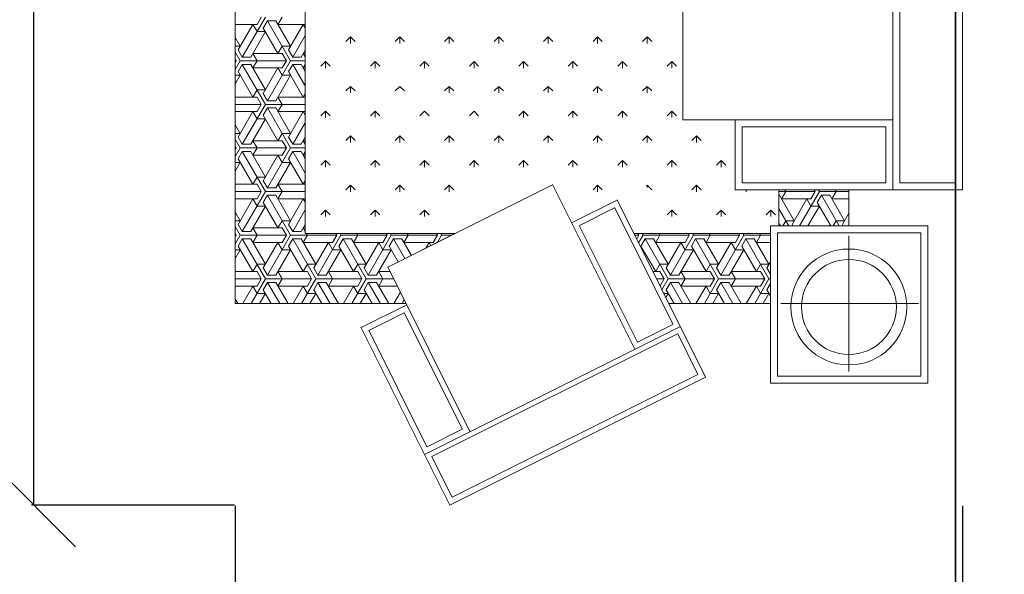
# Model space of a CAD drawing. Units: inches. Extents: x -1198 to -69, y -512 to 437.
# Tile 44 of 50: x -444 to -373, y 5 to 45. Entities that reach past the tile are written whole.
import ezdxf

# ---------------------------------------------------------------- set-up
doc = ezdxf.new("R2010")
doc.units = ezdxf.units.IN
doc.header["$MEASUREMENT"] = 0
for name, color, linetype, lineweight in [('A-ANNO-DIMS', 2, 'Continuous', 18), ('A-FURN', 60, 'Continuous', 18), ('A-WALL', 7, 'Continuous', 35)]:
    doc.layers.add(name, color=color, linetype=linetype, lineweight=lineweight)
doc.styles.get("Standard").update_dxf_attribs({"font": 'arial.ttf'})
doc.dimstyles.get("Standard").update_dxf_attribs({"dimtxt": 6, "dimasz": 6, "dimexe": 0.18, "dimexo": 0.0625, "dimgap": 0.09, "dimtad": 0, "dimtih": 1, "dimtoh": 1, "dimdec": 0, "dimzin": 0, "dimdsep": 46, "dimlunit": 4, "dimtxsty": 'Standard', "dimblk": 'OBLIQUE', "dimcen": 0.09, "dimadec": 0, "dimazin": 0, "dimtfac": 1, "dimtdec": 0, "dimtofl": 0, "dimtmove": 0, "dimatfit": 3, "dimfxl": 1, "dimtolj": 1, "dimtzin": 0, "dimarcsym": 0})

# ---------------------------------------------------------------- blocks, each defined once
blk = doc.blocks.new('A$C3B9F700E')
for p, q in [((736.9, 2080, -685.7), (2936.9, 2080, -685.7)), ((756.9, 2060, -685.7), (2916.9, 2060, -685.7)), ((2916.9, 2060, -685.7), (2916.9, 1900, -685.7)), ((2936.9, 2080, -685.7), (2936.9, 1430, -685.7)), ((2936.9, 2080, -685.7), (2936.9, 1880, -685.7)), ((3489.8, 1980.6, -685.7), (3039.8, 1980.6, -685.7)), ((3039.8, 1980.6, -685.7), (3039.8, 1530.6, -685.7)), ((3489.8, 1530.6, -685.7), (3489.8, 1980.6, -685.7)), ((3469.8, 1960.6, -685.7), (3059.8, 1960.6, -685.7)), ((3059.8, 1960.6, -685.7), (3059.8, 1550.6, -685.7)), ((3262.1, 1953.9, -685.7), (3262.1, 1560.5, -685.7)), ((3469.8, 1550.6, -685.7), (3469.8, 1960.6, -685.7)), ((2916.9, 1900, -685.7), (756.9, 1900, -685.7)), ((2936.9, 1880, -685.7), (736.9, 1880, -685.7)), ((2936.9, 1880, -685.7), (736.9, 1880, -685.7)), ((2736.9, 1880, -685.7), (2736.9, 1280, -685.7)), ((2736.9, 1430, -685.7), (2736.9, 1880, -685.7)), ((2736.9, 1880, -685.7), (2936.9, 1880, -685.7)), ((2756.9, 1450, -685.7), (2756.9, 1860, -685.7)), ((2756.9, 1860, -685.7), (2916.9, 1860, -685.7)), ((2916.9, 1860, -685.7), (2916.9, 1450, -685.7)), ((2936.9, 1880, -685.7), (2936.9, 1430, -685.7)), ((2936.9, 1754.8, -685.7), (3039.8, 1754.8, -685.7)), ((2936.9, 1554.8, -685.7), (2936.9, 1754.8, -685.7)), ((2936.9, 1754.8, -685.7), (3039.8, 1754.8, -685.7)), ((2941.9, 1670.3, -685.7), (2941.9, 1754.8, -685.7)), ((2962.7, 1754.8, -685.7), (2962.7, 1706.3, -685.7)), ((3035.5, 1736.3, -685.7), (3003.4, 1754.8, -685.7)), ((3039.8, 1754.8, -685.7), (3039.8, 1554.8, -685.7)), ((3456.2, 1754.8, -685.7), (3068, 1754.8, -685.7)), ((2941.9, 1718.3, -685.7), (2936.9, 1715.4, -685.7)), ((2941.9, 1718.3, -685.7), (2962.7, 1706.3, -685.7)), ((2952.3, 1700.3, -685.7), (3025.1, 1742.3, -685.7)), ((3039.8, 1726.8, -685.7), (2952.3, 1676.3, -685.7)), ((3025.1, 1718.3, -685.7), (3025.1, 1742.3, -685.7)), ((3025.1, 1718.3, -685.7), (3039.8, 1709.8, -685.7)), ((3039.8, 1738.8, -685.7), (3035.5, 1736.3, -685.7)), ((2952.3, 1676.3, -685.7), (2952.3, 1700.3, -685.7)), ((2973.1, 1664.3, -685.7), (3039.8, 1702.8, -685.7)), ((2941.9, 1670.3, -685.7), (2936.9, 1667.4, -685.7)), ((2941.9, 1670.3, -685.7), (3039.8, 1613.8, -685.7)), ((2952.3, 1676.3, -685.7), (2973.1, 1664.3, -685.7)), ((3039.8, 1637.8, -685.7), (2983.5, 1670.3, -685.7)), ((2983.5, 1646.3, -685.7), (2983.5, 1670.3, -685.7)), ((2941.9, 1658.3, -685.7), (2936.9, 1655.4, -685.7)), ((2941.9, 1658.3, -685.7), (2962.7, 1646.3, -685.7)), ((2941.9, 1554.8, -685.7), (2941.9, 1658.3, -685.7)), ((2962.7, 1646.3, -685.7), (2962.7, 1562.3, -685.7)), ((2983.5, 1646.3, -685.7), (2962.7, 1634.3, -685.7)), ((3035.5, 1592.3, -685.7), (2962.7, 1634.3, -685.7)), ((2952.3, 1556.3, -685.7), (3025.1, 1598.3, -685.7)), ((3039.8, 1582.8, -685.7), (2991.3, 1554.8, -685.7)), ((3025.1, 1574.3, -685.7), (3025.1, 1598.3, -685.7)), ((3039.8, 1594.8, -685.7), (3035.5, 1592.3, -685.7)), ((2941.9, 1574.3, -685.7), (2936.9, 1571.4, -685.7)), ((3039.8, 1554.8, -685.7), (2936.9, 1554.8, -685.7)), ((2936.9, 1554.8, -685.7), (3039.8, 1554.8, -685.7)), ((2941.9, 1574.3, -685.7), (2962.7, 1562.3, -685.7)), ((2952.3, 1554.8, -685.7), (2952.3, 1556.3, -685.7)), ((3025.1, 1574.3, -685.7), (3039.8, 1565.8, -685.7)), ((3032.8, 1554.8, -685.7), (3039.8, 1558.8, -685.7)), ((3059.8, 1550.6, -685.7), (3469.8, 1550.6, -685.7)), ((2994.6, 1531.3, -685.7), (3007.9, 1544.5, -685.7)), ((2994.6, 1531.3, -685.7), (3013.4, 1531.3, -685.7)), ((2994.6, 1531.3, -685.7), (3007.9, 1518, -685.7)), ((3039.8, 1530.6, -685.7), (3489.8, 1530.6, -685.7)), ((3062.1, 1140.2, -685.7), (3062.1, 1530.6, -685.7)), ((3062.1, 1530.6, -685.7), (3062.1, 1140.2, -685.7)), ((3062.1, 1530.6, -685.7), (3262.1, 1530.6, -685.7)), ((3066.6, 1454.3, -685.7), (3066.6, 1530.6, -685.7)), ((3077, 1484.3, -685.7), (3149.8, 1526.3, -685.7)), ((3191.3, 1526.3, -685.7), (3077, 1460.3, -685.7)), ((3087.4, 1530.6, -685.7), (3087.4, 1490.3, -685.7)), ((3160.2, 1520.3, -685.7), (3142.3, 1530.6, -685.7)), ((3149.8, 1502.3, -685.7), (3149.8, 1526.3, -685.7)), ((3178, 1530.6, -685.7), (3160.2, 1520.3, -685.7)), ((3191.3, 1526.3, -685.7), (3191.3, 1530.6, -685.7)), ((3191.3, 1526.3, -685.7), (3262.1, 1485.5, -685.7)), ((3204.7, 1530.6, -685.7), (3222.5, 1520.3, -685.7)), ((3222.5, 1520.3, -685.7), (3240.3, 1530.6, -685.7)), ((3262.1, 1509.5, -685.7), (3232.9, 1526.3, -685.7)), ((3232.9, 1502.3, -685.7), (3232.9, 1526.3, -685.7)), ((3262.1, 1530.6, -685.7), (3262.1, 1240.1, -685.7)), ((3262.1, 1530.6, -685.7), (3262.1, 1240.1, -685.7)), ((3066.6, 1502.3, -685.7), (3062.1, 1499.7, -685.7)), ((3066.6, 1502.3, -685.7), (3087.4, 1490.3, -685.7)), ((3149.8, 1502.3, -685.7), (3170.6, 1490.3, -685.7)), ((3191.3, 1514.3, -685.7), (3170.6, 1502.3, -685.7)), ((3170.6, 1502.3, -685.7), (3170.6, 1418.3, -685.7)), ((3191.3, 1382.3, -685.7), (3191.3, 1514.3, -685.7)), ((3191.3, 1514.3, -685.7), (3212.1, 1502.3, -685.7)), ((3212.1, 1502.3, -685.7), (3212.1, 1418.3, -685.7)), ((3232.9, 1502.3, -685.7), (3212.1, 1490.3, -685.7)), ((2936.9, 1473.6, -685.7), (2937.2, 1473.8, -685.7)), ((3077, 1460.3, -685.7), (3077, 1484.3, -685.7)), ((3097.8, 1448.3, -685.7), (3170.6, 1490.3, -685.7)), ((3262.1, 1461.5, -685.7), (3212.1, 1490.3, -685.7)), ((2916.9, 1450, -685.7), (2756.9, 1450, -685.7)), ((2936.9, 1460.6, -685.7), (2942.6, 1460.6, -685.7)), ((2936.9, 1447.6, -685.7), (2937.2, 1447.3, -685.7)), ((3066.6, 1454.3, -685.7), (3062.1, 1451.7, -685.7)), ((3066.6, 1442.3, -685.7), (3062.1, 1439.7, -685.7)), ((3066.6, 1454.3, -685.7), (3181, 1388.3, -685.7)), ((3066.6, 1310.3, -685.7), (3066.6, 1442.3, -685.7)), ((3066.6, 1442.3, -685.7), (3087.4, 1430.3, -685.7)), ((3077, 1460.3, -685.7), (3097.8, 1448.3, -685.7)), ((3181, 1412.3, -685.7), (3108.2, 1454.3, -685.7)), ((3108.2, 1430.3, -685.7), (3108.2, 1454.3, -685.7)), ((3201.7, 1412.3, -685.7), (3262.1, 1447.2, -685.7)), ((2936.9, 1430, -685.7), (2736.9, 1430, -685.7)), ((2936.9, 1430, -685.7), (2736.9, 1430, -685.7)), ((3087.4, 1430.3, -685.7), (3087.4, 1346.3, -685.7)), ((3108.2, 1430.3, -685.7), (3087.4, 1418.3, -685.7)), ((3160.2, 1376.3, -685.7), (3087.4, 1418.3, -685.7)), ((3191.3, 1430.3, -685.7), (3170.6, 1418.3, -685.7)), ((3181, 1388.3, -685.7), (3181, 1412.3, -685.7)), ((3191.3, 1430.3, -685.7), (3212.1, 1418.3, -685.7)), ((3262.1, 1423.2, -685.7), (3201.7, 1388.3, -685.7)), ((3201.7, 1388.3, -685.7), (3201.7, 1412.3, -685.7)), ((2853.2, 1389.9, -685.7), (2866.4, 1403.1, -685.7)), ((2853.2, 1389.9, -685.7), (2871.9, 1389.9, -685.7)), ((2853.2, 1389.9, -685.7), (2866.4, 1376.6, -685.7)), ((2994.6, 1389.9, -685.7), (3007.9, 1403.1, -685.7)), ((2994.6, 1389.9, -685.7), (3013.4, 1389.9, -685.7)), ((2994.6, 1389.9, -685.7), (3007.9, 1376.6, -685.7)), ((3077, 1340.3, -685.7), (3149.8, 1382.3, -685.7)), ((3191.3, 1382.3, -685.7), (3077, 1316.3, -685.7)), ((3149.8, 1358.3, -685.7), (3149.8, 1382.3, -685.7)), ((3181, 1388.3, -685.7), (3160.2, 1376.3, -685.7)), ((3191.3, 1382.3, -685.7), (3262.1, 1341.5, -685.7)), ((3201.7, 1388.3, -685.7), (3222.5, 1376.3, -685.7)), ((3222.5, 1376.3, -685.7), (3262.1, 1399.2, -685.7)), ((3262.1, 1365.5, -685.7), (3232.9, 1382.3, -685.7)), ((3232.9, 1358.3, -685.7), (3232.9, 1382.3, -685.7)), ((3066.6, 1358.3, -685.7), (3062.1, 1355.7, -685.7)), ((3066.6, 1358.3, -685.7), (3087.4, 1346.3, -685.7)), ((3149.8, 1358.3, -685.7), (3170.6, 1346.3, -685.7)), ((3191.3, 1370.3, -685.7), (3170.6, 1358.3, -685.7)), ((3170.6, 1358.3, -685.7), (3170.6, 1274.3, -685.7)), ((3191.3, 1370.3, -685.7), (3212.1, 1358.3, -685.7)), ((3191.3, 1238.3, -685.7), (3191.3, 1370.3, -685.7)), ((3212.1, 1358.3, -685.7), (3212.1, 1274.3, -685.7)), ((3232.9, 1358.3, -685.7), (3212.1, 1346.3, -685.7)), ((2782.5, 1319.2, -685.7), (2795.7, 1332.4, -685.7)), ((2923.9, 1319.2, -685.7), (2937.2, 1332.4, -685.7)), ((2965.3, 1091.9, -685.7), (3472.5, 1345.2, -685.7)), ((3077, 1316.3, -685.7), (3077, 1340.3, -685.7)), ((3097.8, 1304.3, -685.7), (3170.6, 1346.3, -685.7)), ((3262.1, 1317.5, -685.7), (3212.1, 1346.3, -685.7)), ((3472.5, 1345.2, -685.7), (3838, 613.2, -685.7)), ((2782.5, 1319.2, -685.7), (2801.2, 1319.2, -685.7)), ((2782.5, 1319.2, -685.7), (2795.7, 1305.9, -685.7)), ((2923.9, 1319.2, -685.7), (2937.2, 1305.9, -685.7)), ((2923.9, 1319.2, -685.7), (2942.6, 1319.2, -685.7)), ((3066.6, 1310.3, -685.7), (3062.1, 1307.7, -685.7)), ((3066.6, 1298.3, -685.7), (3062.1, 1295.7, -685.7)), ((3066.6, 1310.3, -685.7), (3181, 1244.3, -685.7)), ((3066.6, 1298.3, -685.7), (3087.4, 1286.3, -685.7)), ((3066.6, 1166.3, -685.7), (3066.6, 1298.3, -685.7)), ((3077, 1316.3, -685.7), (3097.8, 1304.3, -685.7)), ((3181, 1268.3, -685.7), (3108.2, 1310.3, -685.7)), ((3108.2, 1286.3, -685.7), (3108.2, 1310.3, -685.7)), ((3201.7, 1268.3, -685.7), (3262.1, 1303.2, -685.7)), ((3348.8, 1265.3, -685.7), (3464.4, 1323, -685.7)), ((3464.4, 1323, -685.7), (3815.2, 620.4, -685.7)), ((2736.9, 1280, -685.7), (936.9, 1280, -685.7)), ((3087.4, 1286.3, -685.7), (3087.4, 1202.3, -685.7)), ((3108.2, 1286.3, -685.7), (3087.4, 1274.3, -685.7)), ((3160.2, 1232.3, -685.7), (3087.4, 1274.3, -685.7)), ((3191.3, 1286.3, -685.7), (3170.6, 1274.3, -685.7)), ((3181, 1244.3, -685.7), (3181, 1268.3, -685.7)), ((3191.3, 1286.3, -685.7), (3212.1, 1274.3, -685.7)), ((3262.1, 1279.2, -685.7), (3201.7, 1244.3, -685.7)), ((3201.7, 1244.3, -685.7), (3201.7, 1268.3, -685.7)), ((3327.6, 1272.8, -685.7), (3693.1, 540.9, -685.7)), ((2570.3, 1248.4, -685.7), (2583.6, 1261.7, -685.7)), ((2570.3, 1248.4, -685.7), (2589.1, 1248.4, -685.7)), ((2570.3, 1248.4, -685.7), (2583.6, 1235.2, -685.7)), ((2711.8, 1248.4, -685.7), (2725, 1261.7, -685.7)), ((2711.8, 1248.4, -685.7), (2725, 1235.2, -685.7)), ((2711.8, 1248.4, -685.7), (2730.5, 1248.4, -685.7)), ((2853.2, 1248.4, -685.7), (2866.4, 1261.7, -685.7)), ((2853.2, 1248.4, -685.7), (2866.4, 1235.2, -685.7)), ((2853.2, 1248.4, -685.7), (2871.9, 1248.4, -685.7)), ((2987.4, 1084.8, -685.7), (3320, 1250.9, -685.7)), ((2994.6, 1248.4, -685.7), (3007.9, 1261.7, -685.7)), ((2994.6, 1248.4, -685.7), (3007.9, 1235.2, -685.7)), ((2994.6, 1248.4, -685.7), (3013.4, 1248.4, -685.7)), ((3262.1, 1240.1, -685.7), (3062.1, 1140.2, -685.7)), ((3181, 1244.3, -685.7), (3160.2, 1232.3, -685.7)), ((3201.7, 1244.3, -685.7), (3222.5, 1232.3, -685.7)), ((3222.5, 1232.3, -685.7), (3262.1, 1255.2, -685.7)), ((3321.4, 1251.2, -685.7), (3371.9, 1150.1, -685.7)), ((3348.6, 1264.7, -685.7), (3348.8, 1265.3, -685.7)), ((3699.2, 562.5, -685.7), (3348.6, 1264.7, -685.7)), ((3066.6, 1214.3, -685.7), (3062.1, 1211.7, -685.7)), ((3066.6, 1214.3, -685.7), (3087.4, 1202.3, -685.7)), ((3077, 1196.3, -685.7), (3149.8, 1238.3, -685.7)), ((3191.3, 1238.3, -685.7), (3077, 1172.3, -685.7)), ((3149.8, 1214.3, -685.7), (3149.8, 1238.3, -685.7)), ((3149.8, 1214.3, -685.7), (3170.6, 1202.3, -685.7)), ((3191.3, 1226.3, -685.7), (3170.6, 1214.3, -685.7)), ((3170.6, 1214.3, -685.7), (3170.6, 1194.4, -685.7)), ((3191.3, 1238.3, -685.7), (3222.5, 1220.3, -685.7)), ((3191.3, 1226.3, -685.7), (3211.4, 1214.8, -685.7)), ((3191.3, 1204.8, -685.7), (3191.3, 1226.3, -685.7)), ((3244.8, 1231.5, -685.7), (3232.9, 1238.3, -685.7)), ((3232.9, 1225.5, -685.7), (3232.9, 1238.3, -685.7)), ((2499.6, 1177.7, -685.7), (2512.9, 1191, -685.7)), ((2641.1, 1177.7, -685.7), (2654.3, 1191, -685.7)), ((2782.5, 1177.7, -685.7), (2795.7, 1191, -685.7)), ((2923.9, 1177.7, -685.7), (2937.2, 1191, -685.7)), ((3077, 1172.3, -685.7), (3077, 1196.3, -685.7)), ((3097.8, 1160.3, -685.7), (3170.6, 1202.3, -685.7)), ((2499.6, 1177.7, -685.7), (2512.9, 1164.5, -685.7)), ((2499.6, 1177.7, -685.7), (2518.4, 1177.7, -685.7)), ((2641.1, 1177.7, -685.7), (2654.3, 1164.5, -685.7)), ((2641.1, 1177.7, -685.7), (2659.8, 1177.7, -685.7)), ((2782.5, 1177.7, -685.7), (2801.2, 1177.7, -685.7)), ((2782.5, 1177.7, -685.7), (2795.7, 1164.5, -685.7)), ((2923.9, 1177.7, -685.7), (2925.9, 1175.7, -685.7)), ((2923.9, 1177.7, -685.7), (2930, 1177.7, -685.7)), ((3066.6, 1166.3, -685.7), (3062.1, 1163.7, -685.7)), ((3066.6, 1166.3, -685.7), (3088.8, 1153.5, -685.7)), ((3077, 1172.3, -685.7), (3097.8, 1160.3, -685.7)), ((3111.1, 1164.7, -685.7), (3108.2, 1166.3, -685.7)), ((3108.2, 1163.2, -685.7), (3108.2, 1166.3, -685.7)), ((2921.7, 907.1, -685.7), (3392.7, 1142.3, -685.7)), ((3038.9, 983.8, -685.7), (3371.9, 1150.1, -685.7)), ((3066.6, 1154.3, -685.7), (3062.1, 1151.7, -685.7)), ((3066.6, 1154.3, -685.7), (3077.6, 1148, -685.7)), ((3066.6, 1142.5, -685.7), (3066.6, 1154.3, -685.7)), ((2570.3, 1107, -685.7), (2583.6, 1120.3, -685.7)), ((2570.3, 1107, -685.7), (2589.1, 1107, -685.7)), ((2570.3, 1107, -685.7), (2583.6, 1093.8, -685.7)), ((2711.8, 1107, -685.7), (2725, 1120.3, -685.7)), ((2711.8, 1107, -685.7), (2725, 1093.8, -685.7)), ((2711.8, 1107, -685.7), (2730.5, 1107, -685.7)), ((2853.2, 1107, -685.7), (2866.4, 1120.3, -685.7)), ((2853.2, 1107, -685.7), (2866.4, 1093.8, -685.7)), ((2853.2, 1107, -685.7), (2871.9, 1107, -685.7)), ((2966.2, 1092.3, -685.7), (3031.3, 961.9, -685.7)), ((2988.1, 1084.7, -685.7), (3038.4, 984, -685.7)), ((2499.6, 1036.3, -685.7), (2512.9, 1049.6, -685.7)), ((2641.1, 1036.3, -685.7), (2654.3, 1049.6, -685.7)), ((2782.5, 1036.3, -685.7), (2795.7, 1049.6, -685.7)), ((2923.9, 1036.3, -685.7), (2937.2, 1049.6, -685.7)), ((2499.6, 1036.3, -685.7), (2512.9, 1023.1, -685.7)), ((2499.6, 1036.3, -685.7), (2518.4, 1036.3, -685.7)), ((2641.1, 1036.3, -685.7), (2654.3, 1023.1, -685.7)), ((2641.1, 1036.3, -685.7), (2659.8, 1036.3, -685.7)), ((2782.5, 1036.3, -685.7), (2801.2, 1036.3, -685.7)), ((2782.5, 1036.3, -685.7), (2795.7, 1023.1, -685.7)), ((2923.9, 1036.3, -685.7), (2937.2, 1023.1, -685.7)), ((2923.9, 1036.3, -685.7), (2942.6, 1036.3, -685.7)), ((2570.3, 965.6, -685.7), (2583.6, 978.9, -685.7)), ((2570.3, 965.6, -685.7), (2589.1, 965.6, -685.7)), ((2570.3, 965.6, -685.7), (2583.6, 952.3, -685.7)), ((2711.8, 965.6, -685.7), (2725, 978.9, -685.7)), ((2711.8, 965.6, -685.7), (2725, 952.3, -685.7)), ((2711.8, 965.6, -685.7), (2730.5, 965.6, -685.7)), ((2853.2, 965.6, -685.7), (2866.4, 978.9, -685.7)), ((2853.2, 965.6, -685.7), (2866.4, 952.3, -685.7)), ((2853.2, 965.6, -685.7), (2871.9, 965.6, -685.7)), ((2499.6, 894.9, -685.7), (2512.9, 908.1, -685.7)), ((2641.1, 894.9, -685.7), (2654.3, 908.1, -685.7)), ((2782.5, 894.9, -685.7), (2795.7, 908.1, -685.7)), ((2922.6, 907.6, -685.7), (3157.8, 436.6, -685.7)), ((2499.6, 894.9, -685.7), (2512.9, 881.6, -685.7)), ((2499.6, 894.9, -685.7), (2518.4, 894.9, -685.7)), ((2641.1, 894.9, -685.7), (2654.3, 881.6, -685.7)), ((2641.1, 894.9, -685.7), (2659.8, 894.9, -685.7)), ((2782.5, 894.9, -685.7), (2801.2, 894.9, -685.7)), ((2782.5, 894.9, -685.7), (2795.7, 881.6, -685.7)), ((2570.3, 824.2, -685.7), (2583.6, 837.4, -685.7)), ((2570.3, 824.2, -685.7), (2589.1, 824.2, -685.7)), ((2570.3, 824.2, -685.7), (2583.6, 810.9, -685.7)), ((2711.8, 824.2, -685.7), (2725, 837.4, -685.7)), ((2711.8, 824.2, -685.7), (2725, 810.9, -685.7)), ((2711.8, 824.2, -685.7), (2730.5, 824.2, -685.7)), ((2853.2, 824.2, -685.7), (2866.4, 837.4, -685.7)), ((2853.2, 824.2, -685.7), (2866.4, 810.9, -685.7)), ((2853.2, 824.2, -685.7), (2871.9, 824.2, -685.7)), ((2499.6, 753.5, -685.7), (2512.9, 766.7, -685.7)), ((2641.1, 753.5, -685.7), (2654.3, 766.7, -685.7)), ((2782.5, 753.5, -685.7), (2795.7, 766.7, -685.7)), ((2499.6, 753.5, -685.7), (2512.9, 740.2, -685.7)), ((2499.6, 753.5, -685.7), (2518.4, 753.5, -685.7)), ((2641.1, 753.5, -685.7), (2654.3, 740.2, -685.7)), ((2641.1, 753.5, -685.7), (2659.8, 753.5, -685.7)), ((2782.5, 753.5, -685.7), (2801.2, 753.5, -685.7)), ((2782.5, 753.5, -685.7), (2795.7, 740.2, -685.7)), ((2570.3, 682.8, -685.7), (2583.6, 696, -685.7)), ((2570.3, 682.8, -685.7), (2589.1, 682.8, -685.7)), ((2570.3, 682.8, -685.7), (2583.6, 669.5, -685.7)), ((2711.8, 682.8, -685.7), (2725, 696, -685.7)), ((2711.8, 682.8, -685.7), (2725, 669.5, -685.7)), ((2853.2, 682.8, -685.7), (2866.4, 696, -685.7)), ((2853.2, 682.8, -685.7), (2866.4, 669.5, -685.7)), ((2853.2, 682.8, -685.7), (2871.9, 682.8, -685.7)), ((3156.9, 436.1, -685.7), (3627.9, 671.3, -685.7)), ((3287.7, 483.3, -685.7), (3620.3, 649.4, -685.7)), ((3620.9, 649.2, -685.7), (3671.2, 548.5, -685.7)), ((2499.6, 612, -685.7), (2512.9, 625.3, -685.7)), ((2641.1, 612, -685.7), (2654.3, 625.3, -685.7)), ((2782.5, 612, -685.7), (2795.7, 625.3, -685.7)), ((2923.9, 612, -685.7), (2937.2, 625.3, -685.7)), ((3062.1, 628.3, -685.7), (3062.1, 200, -685.7)), ((3157.8, 436.6, -685.7), (3062.1, 628.3, -685.7)), ((3062.1, 628.3, -685.7), (3062.1, 200, -685.7)), ((3815, 619.9, -685.7), (3699.8, 562.3, -685.7)), ((3815.2, 620.4, -685.7), (3815, 619.9, -685.7)), ((2499.6, 612, -685.7), (2512.9, 598.8, -685.7)), ((2499.6, 612, -685.7), (2518.4, 612, -685.7)), ((2641.1, 612, -685.7), (2654.3, 598.8, -685.7)), ((2641.1, 612, -685.7), (2659.8, 612, -685.7)), ((2782.5, 612, -685.7), (2801.2, 612, -685.7)), ((2782.5, 612, -685.7), (2795.7, 598.8, -685.7)), ((2923.9, 612, -685.7), (2937.2, 598.8, -685.7)), ((2923.9, 612, -685.7), (2942.6, 612, -685.7)), ((3066.6, 590.3, -685.7), (3066.6, 619.2, -685.7)), ((3077, 596.3, -685.7), (3077, 598.3, -685.7)), ((3077.8, 596.8, -685.7), (3077, 596.3, -685.7)), ((3077, 596.3, -685.7), (3078.4, 595.5, -685.7)), ((3329.8, 359.5, -685.7), (3838, 613.2, -685.7)), ((3066.6, 590.3, -685.7), (3062.1, 587.7, -685.7)), ((3066.6, 578.3, -685.7), (3062.1, 575.7, -685.7)), ((3066.6, 590.3, -685.7), (3086.9, 578.6, -685.7)), ((3066.6, 578.3, -685.7), (3087.4, 566.3, -685.7)), ((3066.6, 446.3, -685.7), (3066.6, 578.3, -685.7)), ((3087.4, 566.3, -685.7), (3087.4, 482.3, -685.7)), ((2570.3, 541.3, -685.7), (2583.6, 554.6, -685.7)), ((2570.3, 541.3, -685.7), (2589.1, 541.3, -685.7)), ((2570.3, 541.3, -685.7), (2583.6, 528.1, -685.7)), ((2711.8, 541.3, -685.7), (2725, 554.6, -685.7)), ((2711.8, 541.3, -685.7), (2725, 528.1, -685.7)), ((2853.2, 541.3, -685.7), (2866.4, 554.6, -685.7)), ((2853.2, 541.3, -685.7), (2866.4, 528.1, -685.7)), ((2853.2, 541.3, -685.7), (2871.9, 541.3, -685.7)), ((2994.6, 541.3, -685.7), (3007.9, 554.6, -685.7)), ((2994.6, 541.3, -685.7), (3007.9, 528.1, -685.7)), ((2994.6, 541.3, -685.7), (3013.4, 541.3, -685.7)), ((3096.4, 559.5, -685.7), (3087.4, 554.3, -685.7)), ((3103.7, 544.9, -685.7), (3087.4, 554.3, -685.7)), ((3338.4, 381.8, -685.7), (3671, 547.9, -685.7)), ((3699.8, 562.3, -685.7), (3699.2, 562.5, -685.7)), ((2499.6, 470.6, -685.7), (2512.9, 483.9, -685.7)), ((2641.1, 470.6, -685.7), (2654.3, 483.9, -685.7)), ((2782.5, 470.6, -685.7), (2795.7, 483.9, -685.7)), ((2923.9, 470.6, -685.7), (2937.2, 483.9, -685.7)), ((3066.6, 494.3, -685.7), (3062.1, 491.7, -685.7)), ((3066.6, 494.3, -685.7), (3087.4, 482.3, -685.7)), ((3077, 476.3, -685.7), (3124.3, 503.6, -685.7)), ((3133.6, 485, -685.7), (3077, 452.3, -685.7)), ((3262.1, 488.6, -685.7), (3157.8, 436.6, -685.7)), ((3251.7, 483.5, -685.7), (3262.1, 477.5, -685.7)), ((3262.1, 0, -685.7), (3262.1, 488.6, -685.7)), ((3262.1, 488.6, -685.7), (3262.1, 0, -685.7)), ((3265.6, 490.4, -685.7), (3330.7, 359.9, -685.7)), ((3288.4, 483.2, -685.7), (3338.7, 382.5, -685.7)), ((2499.6, 470.6, -685.7), (2518.4, 470.6, -685.7)), ((2499.6, 470.6, -685.7), (2512.9, 457.4, -685.7)), ((2641.1, 470.6, -685.7), (2654.3, 457.4, -685.7)), ((2782.5, 470.6, -685.7), (2801.2, 470.6, -685.7)), ((2782.5, 470.6, -685.7), (2795.7, 457.4, -685.7)), ((2923.9, 470.6, -685.7), (2942.6, 470.6, -685.7)), ((2923.9, 470.6, -685.7), (2937.2, 457.4, -685.7)), ((3077, 452.3, -685.7), (3077, 476.3, -685.7)), ((3077, 452.3, -685.7), (3097.8, 440.3, -685.7)), ((3097.8, 440.3, -685.7), (3142.9, 466.4, -685.7)), ((3191.3, 374.3, -685.7), (3191.3, 453.3, -685.7)), ((3212.1, 463.7, -685.7), (3212.1, 410.3, -685.7)), ((3262.1, 453.5, -685.7), (3229.4, 472.3, -685.7)), ((3066.6, 446.3, -685.7), (3062.1, 443.7, -685.7)), ((3066.6, 434.3, -685.7), (3062.1, 431.7, -685.7)), ((3066.6, 446.3, -685.7), (3181, 380.3, -685.7)), ((3066.6, 434.3, -685.7), (3087.4, 422.3, -685.7)), ((3066.6, 302.3, -685.7), (3066.6, 434.3, -685.7)), ((3181, 404.3, -685.7), (3108.2, 446.3, -685.7)), ((3108.2, 422.3, -685.7), (3108.2, 446.3, -685.7)), ((3170.6, 442.9, -685.7), (3170.6, 410.3, -685.7)), ((3201.7, 404.3, -685.7), (3262.1, 439.2, -685.7)), ((2570.3, 399.9, -685.7), (2583.6, 413.2, -685.7)), ((2570.3, 399.9, -685.7), (2589.1, 399.9, -685.7)), ((2570.3, 399.9, -685.7), (2583.6, 386.7, -685.7)), ((2711.8, 399.9, -685.7), (2725, 413.2, -685.7)), ((2711.8, 399.9, -685.7), (2730.5, 399.9, -685.7)), ((2711.8, 399.9, -685.7), (2725, 386.7, -685.7)), ((2853.2, 399.9, -685.7), (2866.4, 413.2, -685.7)), ((2853.2, 399.9, -685.7), (2871.9, 399.9, -685.7)), ((2853.2, 399.9, -685.7), (2866.4, 386.7, -685.7)), ((2994.6, 399.9, -685.7), (3007.9, 413.2, -685.7)), ((2994.6, 399.9, -685.7), (3013.4, 399.9, -685.7)), ((2994.6, 399.9, -685.7), (3007.9, 386.7, -685.7)), ((3087.4, 422.3, -685.7), (3087.4, 338.3, -685.7)), ((3108.2, 422.3, -685.7), (3087.4, 410.3, -685.7)), ((3160.2, 368.3, -685.7), (3087.4, 410.3, -685.7)), ((3191.3, 422.3, -685.7), (3170.6, 410.3, -685.7)), ((3181, 380.3, -685.7), (3181, 404.3, -685.7)), ((3191.3, 422.3, -685.7), (3212.1, 410.3, -685.7)), ((3262.1, 415.2, -685.7), (3201.7, 380.3, -685.7)), ((3201.7, 380.3, -685.7), (3201.7, 404.3, -685.7)), ((3077, 332.3, -685.7), (3149.8, 374.3, -685.7)), ((3191.3, 374.3, -685.7), (3077, 308.3, -685.7)), ((3149.8, 350.3, -685.7), (3149.8, 374.3, -685.7)), ((3181, 380.3, -685.7), (3160.2, 368.3, -685.7)), ((3191.3, 374.3, -685.7), (3262.1, 333.5, -685.7)), ((3201.7, 380.3, -685.7), (3222.5, 368.3, -685.7)), ((3222.5, 368.3, -685.7), (3262.1, 391.2, -685.7)), ((3262.1, 357.5, -685.7), (3232.9, 374.3, -685.7)), ((3232.9, 350.3, -685.7), (3232.9, 374.3, -685.7)), ((2499.6, 329.2, -685.7), (2512.9, 342.5, -685.7)), ((2641.1, 329.2, -685.7), (2654.3, 342.5, -685.7)), ((2782.5, 329.2, -685.7), (2795.7, 342.5, -685.7)), ((2923.9, 329.2, -685.7), (2937.2, 342.5, -685.7)), ((3066.6, 350.3, -685.7), (3062.1, 347.7, -685.7)), ((3066.6, 350.3, -685.7), (3087.4, 338.3, -685.7)), ((3097.8, 296.3, -685.7), (3170.6, 338.3, -685.7)), ((3149.8, 350.3, -685.7), (3170.6, 338.3, -685.7)), ((3191.3, 362.3, -685.7), (3170.6, 350.3, -685.7)), ((3170.6, 350.3, -685.7), (3170.6, 266.3, -685.7)), ((3191.3, 362.3, -685.7), (3212.1, 350.3, -685.7)), ((3191.3, 230.3, -685.7), (3191.3, 362.3, -685.7)), ((3212.1, 350.3, -685.7), (3212.1, 266.3, -685.7)), ((3232.9, 350.3, -685.7), (3212.1, 338.3, -685.7)), ((3262.1, 309.5, -685.7), (3212.1, 338.3, -685.7)), ((2499.6, 329.2, -685.7), (2512.9, 315.9, -685.7)), ((2499.6, 329.2, -685.7), (2518.4, 329.2, -685.7)), ((2641.1, 329.2, -685.7), (2654.3, 315.9, -685.7)), ((2641.1, 329.2, -685.7), (2659.8, 329.2, -685.7)), ((2782.5, 329.2, -685.7), (2801.2, 329.2, -685.7)), ((2782.5, 329.2, -685.7), (2795.7, 315.9, -685.7)), ((2923.9, 329.2, -685.7), (2937.2, 315.9, -685.7)), ((2923.9, 329.2, -685.7), (2942.6, 329.2, -685.7)), ((3077, 308.3, -685.7), (3077, 332.3, -685.7)), ((3066.6, 302.3, -685.7), (3062.1, 299.7, -685.7)), ((3066.6, 290.3, -685.7), (3062.1, 287.7, -685.7)), ((3066.6, 302.3, -685.7), (3181, 236.3, -685.7)), ((3066.6, 290.3, -685.7), (3087.4, 278.3, -685.7)), ((3066.6, 158.3, -685.7), (3066.6, 290.3, -685.7)), ((3077, 308.3, -685.7), (3097.8, 296.3, -685.7)), ((3181, 260.3, -685.7), (3108.2, 302.3, -685.7)), ((3108.2, 278.3, -685.7), (3108.2, 302.3, -685.7)), ((3201.7, 260.3, -685.7), (3262.1, 295.2, -685.7)), ((2570.3, 258.5, -685.7), (2583.6, 271.8, -685.7)), ((2570.3, 258.5, -685.7), (2589.1, 258.5, -685.7)), ((2570.3, 258.5, -685.7), (2583.6, 245.2, -685.7)), ((2711.8, 258.5, -685.7), (2725, 271.8, -685.7)), ((2711.8, 258.5, -685.7), (2725, 245.2, -685.7)), ((2711.8, 258.5, -685.7), (2730.5, 258.5, -685.7)), ((2853.2, 258.5, -685.7), (2866.4, 271.8, -685.7)), ((2853.2, 258.5, -685.7), (2866.4, 245.2, -685.7)), ((2853.2, 258.5, -685.7), (2871.9, 258.5, -685.7)), ((2994.6, 258.5, -685.7), (3007.9, 271.8, -685.7)), ((2994.6, 258.5, -685.7), (3007.9, 245.2, -685.7)), ((2994.6, 258.5, -685.7), (3013.4, 258.5, -685.7)), ((3087.4, 278.3, -685.7), (3087.4, 194.3, -685.7)), ((3108.2, 278.3, -685.7), (3087.4, 266.3, -685.7)), ((3160.2, 224.3, -685.7), (3087.4, 266.3, -685.7)), ((3191.3, 278.3, -685.7), (3170.6, 266.3, -685.7)), ((3181, 236.3, -685.7), (3181, 260.3, -685.7)), ((3191.3, 278.3, -685.7), (3212.1, 266.3, -685.7)), ((3262.1, 271.2, -685.7), (3201.7, 236.3, -685.7)), ((3201.7, 236.3, -685.7), (3201.7, 260.3, -685.7)), ((3077, 188.3, -685.7), (3149.8, 230.3, -685.7)), ((3191.3, 230.3, -685.7), (3077, 164.3, -685.7)), ((3149.8, 206.3, -685.7), (3149.8, 230.3, -685.7)), ((3181, 236.3, -685.7), (3160.2, 224.3, -685.7)), ((3191.3, 230.3, -685.7), (3262.1, 189.5, -685.7)), ((3201.7, 236.3, -685.7), (3222.5, 224.3, -685.7)), ((3222.5, 224.3, -685.7), (3262.1, 247.2, -685.7)), ((3262.1, 213.5, -685.7), (3232.9, 230.3, -685.7)), ((3232.9, 206.3, -685.7), (3232.9, 230.3, -685.7)), ((3062.1, 200, -685.7), (601.4, 200, -685.7)), ((3062.1, 200, -685.7), (601.4, 200, -685.7)), ((2463.9, 200, -685.7), (2463.9, 122.3, -685.7)), ((2473.7, 200, -685.7), (2463.9, 194.3, -685.7)), ((2495.6, 200, -685.7), (2557.4, 164.3, -685.7)), ((2511.8, 200, -685.7), (2512.9, 201, -685.7)), ((2557.4, 188.3, -685.7), (2537.2, 200, -685.7)), ((2547, 200, -685.7), (2547, 194.3, -685.7)), ((2556.9, 200, -685.7), (2547, 194.3, -685.7)), ((2567.8, 158.3, -685.7), (2567.8, 200, -685.7)), ((2578.2, 188.3, -685.7), (2598.4, 200, -685.7)), ((2640, 200, -685.7), (2578.2, 164.3, -685.7)), ((2578.8, 200, -685.7), (2588.6, 194.3, -685.7)), ((2588.6, 200, -685.7), (2588.6, 194.3, -685.7)), ((2653.3, 200, -685.7), (2654.3, 201, -685.7)), ((2661.9, 200, -685.7), (2671.7, 194.3, -685.7)), ((2671.7, 200, -685.7), (2671.7, 122.3, -685.7)), ((2692.5, 86.3, -685.7), (2692.5, 200, -685.7)), ((2713.3, 200, -685.7), (2713.3, 122.3, -685.7)), ((2723.1, 200, -685.7), (2713.3, 194.3, -685.7)), ((2745, 200, -685.7), (2806.8, 164.3, -685.7)), ((2806.8, 188.3, -685.7), (2786.6, 200, -685.7)), ((2794.7, 200, -685.7), (2795.7, 201, -685.7)), ((2796.4, 200, -685.7), (2796.4, 194.3, -685.7)), ((2806.3, 200, -685.7), (2796.4, 194.3, -685.7)), ((2817.2, 158.3, -685.7), (2817.2, 200, -685.7)), ((2827.6, 188.3, -685.7), (2847.8, 200, -685.7)), ((2889.4, 200, -685.7), (2827.6, 164.3, -685.7)), ((2828.2, 200, -685.7), (2838, 194.3, -685.7)), ((2838, 200, -685.7), (2838, 194.3, -685.7)), ((2911.3, 200, -685.7), (2921.1, 194.3, -685.7)), ((2921.1, 200, -685.7), (2921.1, 122.3, -685.7)), ((2936.1, 200, -685.7), (2937.2, 201, -685.7)), ((2941.9, 86.3, -685.7), (2941.9, 200, -685.7)), ((2962.7, 200, -685.7), (2962.7, 122.3, -685.7)), ((2972.5, 200, -685.7), (2962.7, 194.3, -685.7)), ((2994.4, 200, -685.7), (3056.2, 164.3, -685.7)), ((3056.2, 188.3, -685.7), (3036, 200, -685.7)), ((3045.9, 200, -685.7), (3045.9, 194.3, -685.7)), ((3055.7, 200, -685.7), (3045.9, 194.3, -685.7)), ((3066.6, 206.3, -685.7), (3062.1, 203.7, -685.7)), ((3066.6, 206.3, -685.7), (3087.4, 194.3, -685.7)), ((3149.8, 206.3, -685.7), (3170.6, 194.3, -685.7)), ((3191.3, 218.3, -685.7), (3170.6, 206.3, -685.7)), ((3170.6, 206.3, -685.7), (3170.6, 122.3, -685.7)), ((3191.3, 218.3, -685.7), (3212.1, 206.3, -685.7)), ((3191.3, 86.3, -685.7), (3191.3, 218.3, -685.7)), ((3212.1, 206.3, -685.7), (3212.1, 122.3, -685.7)), ((3232.9, 206.3, -685.7), (3212.1, 194.3, -685.7)), ((2536.6, 152.3, -685.7), (2463.9, 194.3, -685.7)), ((2557.4, 164.3, -685.7), (2557.4, 188.3, -685.7)), ((2578.2, 164.3, -685.7), (2578.2, 188.3, -685.7)), ((2599, 152.3, -685.7), (2671.7, 194.3, -685.7)), ((2786, 152.3, -685.7), (2713.3, 194.3, -685.7)), ((2806.8, 164.3, -685.7), (2806.8, 188.3, -685.7)), ((2827.6, 164.3, -685.7), (2827.6, 188.3, -685.7)), ((2848.4, 152.3, -685.7), (2921.1, 194.3, -685.7)), ((3035.5, 152.3, -685.7), (2962.7, 194.3, -685.7)), ((3056.2, 164.3, -685.7), (3056.2, 188.3, -685.7)), ((3077, 164.3, -685.7), (3077, 188.3, -685.7)), ((3097.8, 152.3, -685.7), (3170.6, 194.3, -685.7)), ((3262.1, 165.5, -685.7), (3212.1, 194.3, -685.7)), ((2453.5, 116.3, -685.7), (2526.2, 158.3, -685.7)), ((2567.8, 158.3, -685.7), (2453.5, 92.3, -685.7)), ((2526.2, 134.3, -685.7), (2526.2, 158.3, -685.7)), ((2557.4, 164.3, -685.7), (2536.6, 152.3, -685.7)), ((2567.8, 146.3, -685.7), (2547, 134.3, -685.7)), ((2567.8, 158.3, -685.7), (2682.1, 92.3, -685.7)), ((2567.8, 146.3, -685.7), (2588.6, 134.3, -685.7)), ((2567.8, 14.3, -685.7), (2567.8, 146.3, -685.7)), ((2578.2, 164.3, -685.7), (2599, 152.3, -685.7)), ((2682.1, 116.3, -685.7), (2609.4, 158.3, -685.7)), ((2609.4, 134.3, -685.7), (2609.4, 158.3, -685.7)), ((2702.9, 116.3, -685.7), (2775.7, 158.3, -685.7)), ((2817.2, 158.3, -685.7), (2702.9, 92.3, -685.7)), ((2775.7, 134.3, -685.7), (2775.7, 158.3, -685.7)), ((2806.8, 164.3, -685.7), (2786, 152.3, -685.7)), ((2817.2, 146.3, -685.7), (2796.4, 134.3, -685.7)), ((2817.2, 158.3, -685.7), (2931.5, 92.3, -685.7)), ((2817.2, 146.3, -685.7), (2838, 134.3, -685.7)), ((2817.2, 14.3, -685.7), (2817.2, 146.3, -685.7)), ((2827.6, 164.3, -685.7), (2848.4, 152.3, -685.7)), ((2931.5, 116.3, -685.7), (2858.8, 158.3, -685.7)), ((2858.8, 134.3, -685.7), (2858.8, 158.3, -685.7)), ((2952.3, 116.3, -685.7), (3025.1, 158.3, -685.7)), ((3066.6, 158.3, -685.7), (2952.3, 92.3, -685.7)), ((3025.1, 134.3, -685.7), (3025.1, 158.3, -685.7)), ((3056.2, 164.3, -685.7), (3035.5, 152.3, -685.7)), ((3066.6, 146.3, -685.7), (3045.9, 134.3, -685.7)), ((3066.6, 158.3, -685.7), (3181, 92.3, -685.7)), ((3066.6, 146.3, -685.7), (3087.4, 134.3, -685.7)), ((3066.6, 14.3, -685.7), (3066.6, 146.3, -685.7)), ((3077, 164.3, -685.7), (3097.8, 152.3, -685.7)), ((3181, 116.3, -685.7), (3108.2, 158.3, -685.7)), ((3108.2, 134.3, -685.7), (3108.2, 158.3, -685.7)), ((3201.7, 116.3, -685.7), (3262.1, 151.2, -685.7)), ((2443.1, 134.3, -685.7), (2463.9, 122.3, -685.7)), ((2453.5, 92.3, -685.7), (2453.5, 116.3, -685.7)), ((2474.3, 80.3, -685.7), (2547, 122.3, -685.7)), ((2526.2, 134.3, -685.7), (2547, 122.3, -685.7)), ((2547, 134.3, -685.7), (2547, 50.3, -685.7)), ((2588.6, 134.3, -685.7), (2588.6, 50.3, -685.7)), ((2609.4, 134.3, -685.7), (2588.6, 122.3, -685.7)), ((2661.3, 80.3, -685.7), (2588.6, 122.3, -685.7)), ((2692.5, 134.3, -685.7), (2671.7, 122.3, -685.7)), ((2682.1, 92.3, -685.7), (2682.1, 116.3, -685.7)), ((2692.5, 134.3, -685.7), (2713.3, 122.3, -685.7)), ((2702.9, 92.3, -685.7), (2702.9, 116.3, -685.7)), ((2723.7, 80.3, -685.7), (2796.4, 122.3, -685.7)), ((2775.7, 134.3, -685.7), (2796.4, 122.3, -685.7)), ((2796.4, 134.3, -685.7), (2796.4, 50.3, -685.7)), ((2838, 134.3, -685.7), (2838, 50.3, -685.7)), ((2858.8, 134.3, -685.7), (2838, 122.3, -685.7)), ((2910.8, 80.3, -685.7), (2838, 122.3, -685.7)), ((2941.9, 134.3, -685.7), (2921.1, 122.3, -685.7)), ((2931.5, 92.3, -685.7), (2931.5, 116.3, -685.7)), ((2941.9, 134.3, -685.7), (2962.7, 122.3, -685.7)), ((2952.3, 92.3, -685.7), (2952.3, 116.3, -685.7)), ((2973.1, 80.3, -685.7), (3045.9, 122.3, -685.7)), ((3025.1, 134.3, -685.7), (3045.9, 122.3, -685.7)), ((3045.9, 134.3, -685.7), (3045.9, 50.3, -685.7)), ((3087.4, 134.3, -685.7), (3087.4, 50.3, -685.7)), ((3108.2, 134.3, -685.7), (3087.4, 122.3, -685.7)), ((3160.2, 80.3, -685.7), (3087.4, 122.3, -685.7)), ((3191.3, 134.3, -685.7), (3170.6, 122.3, -685.7)), ((3181, 92.3, -685.7), (3181, 116.3, -685.7)), ((3191.3, 134.3, -685.7), (3212.1, 122.3, -685.7)), ((3262.1, 127.2, -685.7), (3201.7, 92.3, -685.7)), ((3201.7, 92.3, -685.7), (3201.7, 116.3, -685.7)), ((2443.1, 86.3, -685.7), (2557.4, 20.3, -685.7)), ((2453.5, 92.3, -685.7), (2474.3, 80.3, -685.7)), ((2484.7, 62.3, -685.7), (2484.7, 86.3, -685.7)), ((2557.4, 44.3, -685.7), (2484.7, 86.3, -685.7)), ((2578.2, 44.3, -685.7), (2650.9, 86.3, -685.7)), ((2692.5, 86.3, -685.7), (2578.2, 20.3, -685.7)), ((2650.9, 62.3, -685.7), (2650.9, 86.3, -685.7)), ((2682.1, 92.3, -685.7), (2661.3, 80.3, -685.7)), ((2692.5, 86.3, -685.7), (2806.8, 20.3, -685.7)), ((2702.9, 92.3, -685.7), (2723.7, 80.3, -685.7)), ((2806.8, 44.3, -685.7), (2734.1, 86.3, -685.7)), ((2734.1, 62.3, -685.7), (2734.1, 86.3, -685.7)), ((2827.6, 44.3, -685.7), (2900.4, 86.3, -685.7)), ((2941.9, 86.3, -685.7), (2827.6, 20.3, -685.7)), ((2900.4, 62.3, -685.7), (2900.4, 86.3, -685.7)), ((2931.5, 92.3, -685.7), (2910.8, 80.3, -685.7)), ((2941.9, 86.3, -685.7), (3056.2, 20.3, -685.7)), ((2952.3, 92.3, -685.7), (2973.1, 80.3, -685.7)), ((2983.5, 62.3, -685.7), (2983.5, 86.3, -685.7)), ((3056.2, 44.3, -685.7), (2983.5, 86.3, -685.7)), ((3077, 44.3, -685.7), (3149.8, 86.3, -685.7)), ((3191.3, 86.3, -685.7), (3077, 20.3, -685.7)), ((3149.8, 62.3, -685.7), (3149.8, 86.3, -685.7)), ((3181, 92.3, -685.7), (3160.2, 80.3, -685.7)), ((3191.3, 86.3, -685.7), (3262.1, 45.5, -685.7)), ((3201.7, 92.3, -685.7), (3222.5, 80.3, -685.7)), ((3222.5, 80.3, -685.7), (3262.1, 103.2, -685.7)), ((3262.1, 69.5, -685.7), (3232.9, 86.3, -685.7)), ((3232.9, 62.3, -685.7), (3232.9, 86.3, -685.7)), ((2443.1, 74.3, -685.7), (2463.9, 62.3, -685.7)), ((2463.9, 62.3, -685.7), (2463.9, 0, -685.7)), ((2484.7, 62.3, -685.7), (2463.9, 50.3, -685.7)), ((2567.8, 62.3, -685.7), (2547, 50.3, -685.7)), ((2567.8, 62.3, -685.7), (2588.6, 50.3, -685.7)), ((2650.9, 62.3, -685.7), (2671.7, 50.3, -685.7)), ((2692.5, 74.3, -685.7), (2671.7, 62.3, -685.7)), ((2671.7, 62.3, -685.7), (2671.7, 0, -685.7)), ((2692.5, 74.3, -685.7), (2713.3, 62.3, -685.7)), ((2692.5, 0, -685.7), (2692.5, 74.3, -685.7)), ((2713.3, 62.3, -685.7), (2713.3, 0, -685.7)), ((2734.1, 62.3, -685.7), (2713.3, 50.3, -685.7)), ((2817.2, 62.3, -685.7), (2796.4, 50.3, -685.7)), ((2817.2, 62.3, -685.7), (2838, 50.3, -685.7)), ((2900.4, 62.3, -685.7), (2921.1, 50.3, -685.7)), ((2941.9, 74.3, -685.7), (2921.1, 62.3, -685.7)), ((2921.1, 62.3, -685.7), (2921.1, 0, -685.7)), ((2941.9, 74.3, -685.7), (2962.7, 62.3, -685.7)), ((2941.9, 0, -685.7), (2941.9, 74.3, -685.7)), ((2962.7, 62.3, -685.7), (2962.7, 0, -685.7)), ((2983.5, 62.3, -685.7), (2962.7, 50.3, -685.7)), ((3066.6, 62.3, -685.7), (3045.9, 50.3, -685.7)), ((3066.6, 62.3, -685.7), (3087.4, 50.3, -685.7)), ((3149.8, 62.3, -685.7), (3170.6, 50.3, -685.7)), ((3191.3, 74.3, -685.7), (3170.6, 62.3, -685.7)), ((3170.6, 62.3, -685.7), (3170.6, 0, -685.7)), ((3191.3, 74.3, -685.7), (3212.1, 62.3, -685.7)), ((3191.3, 0, -685.7), (3191.3, 74.3, -685.7)), ((3212.1, 62.3, -685.7), (3212.1, 0, -685.7)), ((3232.9, 62.3, -685.7), (3212.1, 50.3, -685.7)), ((2536.6, 8.3, -685.7), (2463.9, 50.3, -685.7)), ((2557.4, 20.3, -685.7), (2557.4, 44.3, -685.7)), ((2578.2, 20.3, -685.7), (2578.2, 44.3, -685.7)), ((2599, 8.3, -685.7), (2671.7, 50.3, -685.7)), ((2786, 8.3, -685.7), (2713.3, 50.3, -685.7)), ((2806.8, 20.3, -685.7), (2806.8, 44.3, -685.7)), ((2827.6, 20.3, -685.7), (2827.6, 44.3, -685.7)), ((2848.4, 8.3, -685.7), (2921.1, 50.3, -685.7)), ((3035.5, 8.3, -685.7), (2962.7, 50.3, -685.7)), ((3056.2, 20.3, -685.7), (3056.2, 44.3, -685.7)), ((3077, 20.3, -685.7), (3077, 44.3, -685.7)), ((3097.8, 8.3, -685.7), (3170.6, 50.3, -685.7)), ((3262.1, 21.5, -685.7), (3212.1, 50.3, -685.7)), ((401.4, 0, -685.7), (3262.1, 0, -685.7)), ((3262.1, 0, -685.7), (401.4, 0, -685.7)), ((2501.4, 0, -685.7), (2526.2, 14.3, -685.7)), ((2526.2, 0, -685.7), (2526.2, 14.3, -685.7)), ((2557.4, 20.3, -685.7), (2536.6, 8.3, -685.7)), ((2567.8, 14.3, -685.7), (2543, 0, -685.7)), ((2567.8, 2.3, -685.7), (2563.8, 0, -685.7)), ((2567.8, 14.3, -685.7), (2592.6, 0, -685.7)), ((2567.8, 2.3, -685.7), (2571.8, 0, -685.7)), ((2567.8, 0, -685.7), (2567.8, 2.3, -685.7)), ((2578.2, 20.3, -685.7), (2599, 8.3, -685.7)), ((2634.2, 0, -685.7), (2609.4, 14.3, -685.7)), ((2609.4, 0, -685.7), (2609.4, 14.3, -685.7)), ((2750.8, 0, -685.7), (2775.7, 14.3, -685.7)), ((2775.7, 0, -685.7), (2775.7, 14.3, -685.7)), ((2806.8, 20.3, -685.7), (2786, 8.3, -685.7)), ((2817.2, 14.3, -685.7), (2792.4, 0, -685.7)), ((2817.2, 2.3, -685.7), (2813.2, 0, -685.7)), ((2817.2, 14.3, -685.7), (2842, 0, -685.7)), ((2817.2, 2.3, -685.7), (2821.2, 0, -685.7)), ((2817.2, 0, -685.7), (2817.2, 2.3, -685.7)), ((2827.6, 20.3, -685.7), (2848.4, 8.3, -685.7)), ((2883.6, 0, -685.7), (2858.8, 14.3, -685.7)), ((2858.8, 0, -685.7), (2858.8, 14.3, -685.7)), ((3000.3, 0, -685.7), (3025.1, 14.3, -685.7)), ((3025.1, 0, -685.7), (3025.1, 14.3, -685.7)), ((3056.2, 20.3, -685.7), (3035.5, 8.3, -685.7)), ((3066.6, 14.3, -685.7), (3041.8, 0, -685.7)), ((3066.6, 2.3, -685.7), (3062.6, 0, -685.7)), ((3066.6, 14.3, -685.7), (3091.4, 0, -685.7)), ((3066.6, 2.3, -685.7), (3070.7, 0, -685.7)), ((3066.6, 0, -685.7), (3066.6, 2.3, -685.7)), ((3077, 20.3, -685.7), (3097.8, 8.3, -685.7)), ((3133, 0, -685.7), (3108.2, 14.3, -685.7)), ((3108.2, 0, -685.7), (3108.2, 14.3, -685.7)), ((3249.7, 0, -685.7), (3262.1, 7.2, -685.7))]:
    blk.add_line(p, q)
for radius in [165.7, 135.7]:
    blk.add_circle((3271.7, 1754.8, -685.7), radius)
blk = doc.blocks.new('1')
blk.add_blockref('A$C3B9F700E', (-1861.1, 172.7, 685.7))
blk = doc.blocks.new('_Oblique')
at = {"color": 0, "linetype": 'ByBlock', "lineweight": -2}
blk.add_line((-0.5, -0.5), (0.5, 0.5), dxfattribs=at)
blk = doc.blocks.new('*D52')
at = {"layer": 'A-ANNO-DIMS', "color": 0, "lineweight": -2, "ltscale": 10, "transparency": 16777216}
for p, q in [((-428.646, 106.551), (-443.249, 106.551)), ((-443.069, 106.551), (-443.069, 61.46)), ((-443.069, 9.981), (-443.069, 55.072)), ((-428.646, 9.981), (-443.249, 9.981))]:
    blk.add_line(p, q, dxfattribs=at)
at = {"layer": 'DEFPOINTS', "color": 0, "ltscale": 10, "transparency": 16777216}
for p in [(-428.584, 106.551), (-443.069, 9.981), (-428.584, 9.981)]:
    blk.add_point(p, dxfattribs=at)
at = {"layer": 'A-ANNO-DIMS', "color": 0, "lineweight": -2, "ltscale": 10, "transparency": 16777216, "xscale": 6, "yscale": 6, "zscale": 6}
for p, rotation in [((-443.069, 106.551), 90), ((-443.069, 9.981), 270)]:
    blk.add_blockref('_Oblique', p, dxfattribs=dict(at, rotation=rotation))
at = {"layer": 'A-ANNO-DIMS', "color": 0, "ltscale": 10, "transparency": 16777216, "insert": (-443.069, 58.266), "char_height": 6, "attachment_point": 5}
blk.add_mtext('\\A1;SEATING GROUP 97 TYP.', dxfattribs=at)
blk = doc.blocks.new('*D53')
at = {"layer": 'A-ANNO-DIMS', "color": 0, "lineweight": -2, "ltscale": 10, "transparency": 16777216}
for p, q in [((-428.584, 9.918), (-428.584, -4.685)), ((-376.248, 9.918), (-376.248, -4.685)), ((-428.584, -4.505), (-417.109, -4.505)), ((-376.248, -4.505), (-387.723, -4.505))]:
    blk.add_line(p, q, dxfattribs=at)
at = {"layer": 'DEFPOINTS', "color": 0, "ltscale": 10, "transparency": 16777216}
for p in [(-428.584, 9.981), (-376.248, 9.981), (-376.248, -4.505)]:
    blk.add_point(p, dxfattribs=at)
at = {"layer": 'A-ANNO-DIMS', "color": 0, "lineweight": -2, "ltscale": 10, "transparency": 16777216, "xscale": 6, "yscale": 6, "zscale": 6, "rotation": 180}
blk.add_blockref('_Oblique', (-428.584, -4.505), dxfattribs=at)
at = {"layer": 'A-ANNO-DIMS', "color": 0, "lineweight": -2, "ltscale": 10, "transparency": 16777216, "xscale": 6, "yscale": 6, "zscale": 6}
blk.add_blockref('_Oblique', (-376.248, -4.505), dxfattribs=at)
at = {"layer": 'A-ANNO-DIMS', "color": 0, "ltscale": 10, "transparency": 16777216, "insert": (-402.416, -4.505), "char_height": 6, "attachment_point": 5}
blk.add_mtext('\\A1;52 TYP.', dxfattribs=at)

msp = doc.modelspace()

# ---------------------------------------------------------------- linework, layer by layer
at = {"layer": 'A-WALL', "ltscale": 10}
msp.add_line((-376.7509, -222.7723), (-376.7509, 257.2277), dxfattribs=at)

# ---------------------------------------------------------------- block references
at = {"layer": 'A-FURN', "ltscale": 10, "xscale": 0.0251614738227896, "yscale": 0.0251614738227896, "zscale": 0.0251614738227896, "rotation": 270.0000000000001}
msp.add_blockref('1', (-432.9284, 59.7223), dxfattribs=at)

# ---------------------------------------------------------------- dimensions: what is measured, and where the dimension line sits
at = {"layer": 'A-ANNO-DIMS', "ltscale": 10}
for base, p1, p2, angle, text, picture, middle in [((-443.0692, 9.981), (-428.5837, 106.551), (-428.5837, 9.981), 270, 'SEATING GROUP <> TYP.', '*D52', (-443.0692, 58.266)), ((-376.2476, -4.5045), (-428.5837, 9.981), (-376.2476, 9.981), 0, '<> TYP.', '*D53', (-402.4157, -4.5045))]:
    dim = msp.add_linear_dim(base=base, p1=p1, p2=p2, angle=angle, text=text, dimstyle='Standard', override={"dimdec": 0, "dimlfac": 1, "dimrnd": 0, "dimzin": 0, "dimdsep": 46, "dimlunit": 2}, dxfattribs=at)
    dim.commit()
    dim.dimension.update_dxf_attribs({"geometry": picture, "text_midpoint": middle})

doc.saveas('drawing.dxf')
